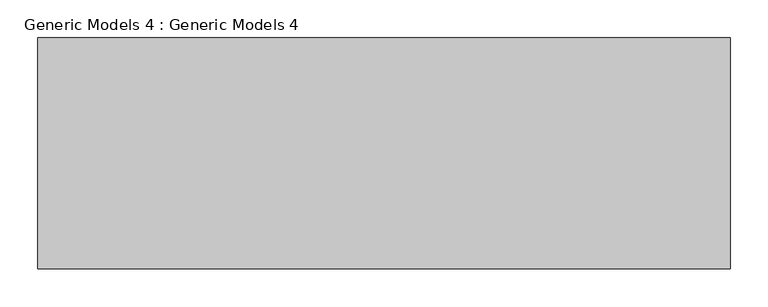
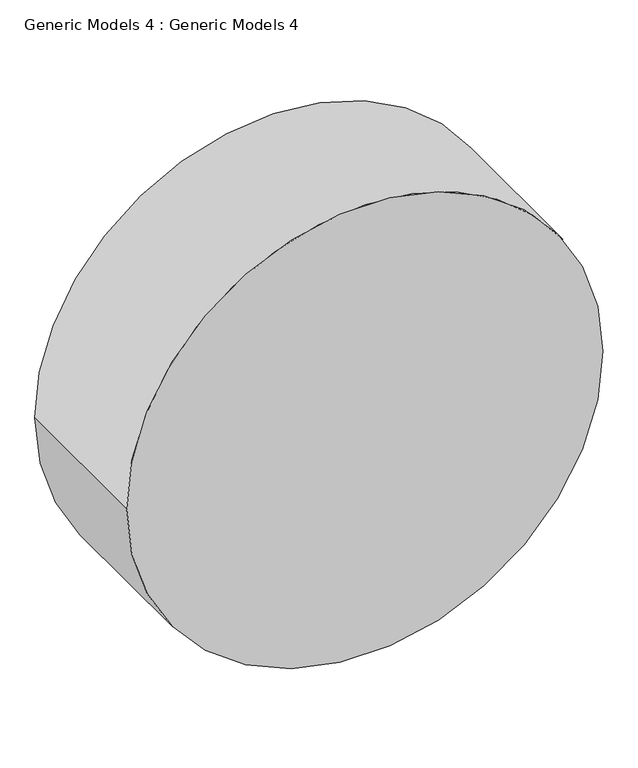
"""IFC4 building model written with IfcOpenShell, lengths in millimetres: proxy geometry, Generic Models 4 : Generic Models 4."""

from ifc_helpers import new_model, si_unit, point, frame, frame_2d, origin, place, context, project, spatial, circle_curve, trimmed, segment, composite_curve, outline, extrude, source, transform, mapped, element, save


def generic_models_4_generic_models_4_0bca1b8b(model_context):
    return source(origin(), model_context, "Body", "SweptSolid", [
        extrude(outline(composite_curve([segment(trimmed(circle_curve(frame_2d((16789.6401483, -1362.7966879)), 457.2), [point((16789.6401483, -1819.9966879))], [point((16789.6401483, -905.5966879))], False, "CARTESIAN"), True, "CONTINUOUS"), segment(trimmed(circle_curve(frame_2d((16789.6401483, -1362.7966879)), 457.2), [point((16789.6401483, -905.5966879))], [point((16789.6401483, -1819.9966879))], False, "CARTESIAN"), True, "CONTINUOUS")], self_intersect=False)), frame((0.0, -2837.5832394, 0.0), z_axis=(0.0, 1.0, 0.0), x_axis=(0.0, 0.0, 1.0)), (0.0, 0.0, 1.0), 304.8),
    ])


if __name__ == "__main__":
    model = new_model("IFC4")
    model_context = context("Model", 3, world=origin())
    ifc_project = project(units=[si_unit("LENGTHUNIT", "METRE", prefix="MILLI")], contexts=[model_context])
    site = spatial("IfcSite", under=ifc_project)
    building = spatial("IfcBuilding", under=site)
    placement = place(None, origin())
    generic_models_4_generic_models_4_shape = generic_models_4_generic_models_4_0bca1b8b(model_context)
    element("IfcBuildingElementProxy", 1, Name="Generic Models 4 : Generic Models 4", ObjectType="Generic Models 4 : Generic Models 4", at=placement, inside=building, context=model_context, shape_type="MappedRepresentation", body=[
        mapped(generic_models_4_generic_models_4_shape, transform((0.0, 0.0, 0.0), x_axis=(1.0, 0.0, 0.0), y_axis=(0.0, 1.0, 0.0), z_axis=(0.0, 0.0, 1.0))),
    ])
    save(model, "model.ifc")

# Revit data of these elements
# Element 1 (IfcBuildingElementProxy, "Generic Models 4 : Generic Models 4")
#   Materials on its faces: "Oak Flooring"
# Materials
#   "Oak Flooring": class "Wood", colour RGB 216 169 114, transparency 0, Description = "Quercus Rubra", Cost = 0
